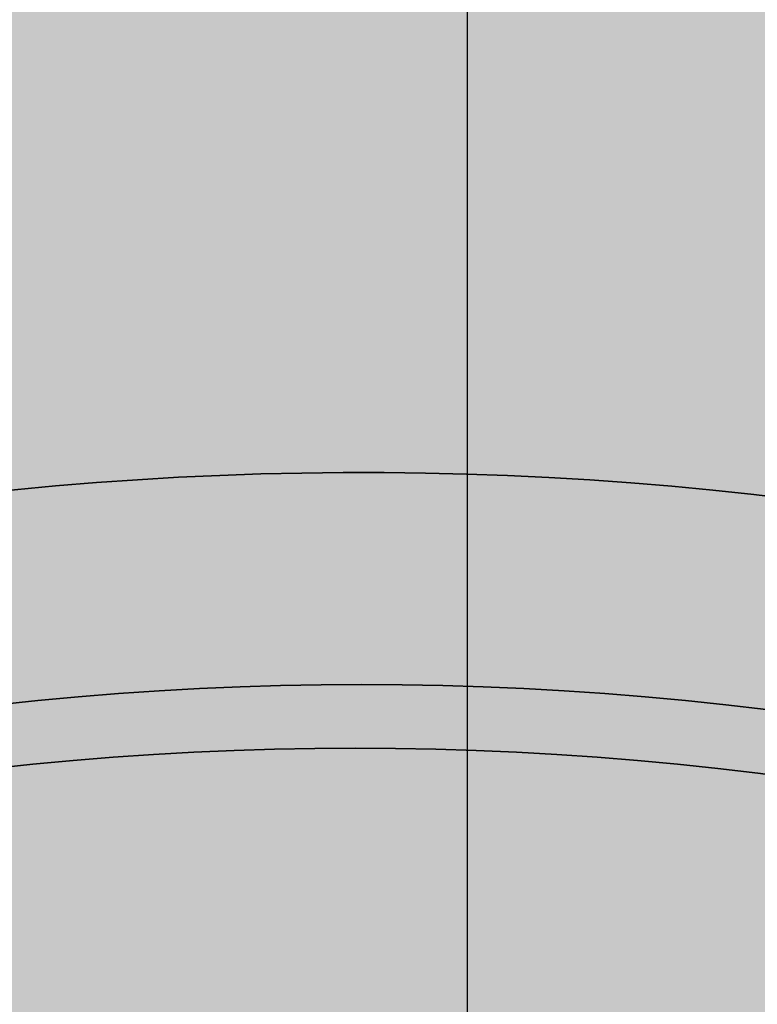
# Model space of a CAD drawing. Units: millimetres. Extents: x 130 to 1021, y 147 to 699.
# Tile 7 of 40: x 411 to 446, y 394 to 440. Entities that reach past the tile are written whole.
import ezdxf

# ---------------------------------------------------------------- set-up
doc = ezdxf.new("R2010")
doc.units = ezdxf.units.MM
doc.header["$MEASUREMENT"] = 0
for name, color, linetype, lineweight in [('A-ANNO-DIMS', 2, 'Continuous', 18), ('A-ELEV', 7, 'Continuous', 35), ('A-ELEV-PATT', 9, 'Continuous', 13)]:
    doc.layers.add(name, color=color, linetype=linetype, lineweight=lineweight)
doc.styles.get("Standard").update_dxf_attribs({"font": 'arial.ttf'})
doc.dimstyles.get("Standard").update_dxf_attribs({"dimtxt": 20, "dimasz": 10, "dimexe": 10, "dimexo": 10, "dimgap": 5, "dimtad": 0, "dimtih": 1, "dimtoh": 1, "dimdec": 0, "dimzin": 0, "dimdsep": 46, "dimtxsty": 'Standard', "dimcen": 5, "dimadec": 0, "dimazin": 0, "dimtfac": 1, "dimtdec": 0, "dimtofl": 0, "dimtmove": 0, "dimatfit": 3, "dimfxl": 1, "dimtolj": 1, "dimtzin": 0, "dimarcsym": 0})

# ---------------------------------------------------------------- blocks, each defined once
blk = doc.blocks.new('*D7')
at = {"layer": 'A-ANNO-DIMS', "color": 0, "lineweight": -2, "transparency": 16777216}
for p, q in [((399.374, 349.447), (413.374, 349.447)), ((423.374, 349.447), (433.374, 349.447)), ((389.374, 344.547), (389.374, 339.447)), ((423.374, 344.547), (423.374, 339.447))]:
    blk.add_line(p, q, dxfattribs=at)
at = {"layer": 'A-ANNO-DIMS', "color": 0, "transparency": 16777216}
for points in [[(399.374, 351.114), (399.374, 347.781), (389.374, 349.447)], [(413.374, 351.114), (413.374, 347.781), (423.374, 349.447)]]:
    blk.add_solid(points, dxfattribs=at)
at = {"layer": 'Defpoints', "color": 0, "transparency": 16777216}
for p in [(389.374, 354.547), (423.374, 354.547), (423.374, 349.447)]:
    blk.add_point(p, dxfattribs=at)
at = {"layer": 'A-ANNO-DIMS', "color": 0, "transparency": 16777216, "insert": (582.037, 349.447), "char_height": 20, "attachment_point": 5}
blk.add_mtext('\\A1;DOOR PANEL 34 TYP.', dxfattribs=at)
blk = doc.blocks.new('*D8')
at = {"layer": 'A-ANNO-DIMS', "color": 0, "lineweight": -2, "transparency": 16777216}
for p, q in [((428.474, 380.947), (428.474, 390.947)), ((428.474, 390.947), (438.474, 390.947)), ((433.374, 370.947), (438.474, 370.947)), ((433.374, 354.547), (438.474, 354.547)), ((428.474, 344.547), (428.474, 334.547))]:
    blk.add_line(p, q, dxfattribs=at)
at = {"layer": 'A-ANNO-DIMS', "color": 0, "transparency": 16777216}
for points in [[(426.807, 380.947), (430.14, 380.947), (428.474, 370.947)], [(426.807, 344.547), (430.14, 344.547), (428.474, 354.547)]]:
    blk.add_solid(points, dxfattribs=at)
at = {"layer": 'Defpoints', "color": 0, "transparency": 16777216}
for p in [(423.374, 370.947), (428.474, 370.947), (423.374, 354.547)]:
    blk.add_point(p, dxfattribs=at)
at = {"layer": 'A-ANNO-DIMS', "color": 0, "transparency": 16777216, "insert": (491.209, 390.947), "char_height": 20, "attachment_point": 5}
blk.add_mtext('\\A1;16 TYP.', dxfattribs=at)
blk = doc.blocks.new('*D11')
at = {"layer": 'A-ANNO-DIMS', "color": 0, "lineweight": -2, "transparency": 16777216}
for p, q in [((737.374, 648.699), (737.374, 149.739)), ((299.374, 566.947), (299.374, 149.739)), ((309.374, 159.739), (490.857, 159.739)), ((727.374, 159.739), (545.891, 159.739))]:
    blk.add_line(p, q, dxfattribs=at)
at = {"layer": 'A-ANNO-DIMS', "color": 0, "transparency": 16777216}
for points in [[(309.374, 161.406), (309.374, 158.073), (299.374, 159.739)], [(727.374, 161.406), (727.374, 158.073), (737.374, 159.739)]]:
    blk.add_solid(points, dxfattribs=at)
at = {"layer": 'Defpoints', "color": 0, "transparency": 16777216}
for p in [(737.374, 658.699), (299.374, 576.947), (737.374, 159.739)]:
    blk.add_point(p, dxfattribs=at)
at = {"layer": 'A-ANNO-DIMS', "color": 0, "transparency": 16777216, "insert": (518.374, 159.739), "char_height": 20, "attachment_point": 5}
blk.add_mtext('\\A1;438', dxfattribs=at)
blk = doc.blocks.new('*D12')
at = {"layer": 'A-ANNO-DIMS', "color": 0, "lineweight": -2, "transparency": 16777216}
for p, q in [((477.374, 661.947), (265.074, 661.947)), ((275.074, 651.947), (275.074, 438.205)), ((275.074, 194.039), (275.074, 407.782)), ((357.163, 184.039), (265.074, 184.039))]:
    blk.add_line(p, q, dxfattribs=at)
at = {"layer": 'A-ANNO-DIMS', "color": 0, "transparency": 16777216}
for points in [[(273.407, 651.947), (276.74, 651.947), (275.074, 661.947)], [(273.407, 194.039), (276.74, 194.039), (275.074, 184.039)]]:
    blk.add_solid(points, dxfattribs=at)
at = {"layer": 'Defpoints', "color": 0, "transparency": 16777216}
for p in [(275.074, 661.947), (487.374, 661.947), (367.163, 184.039)]:
    blk.add_point(p, dxfattribs=at)
at = {"layer": 'A-ANNO-DIMS', "color": 0, "transparency": 16777216, "insert": (275.074, 422.993), "char_height": 20, "attachment_point": 5}
blk.add_mtext('\\A1;477.9', dxfattribs=at)
blk = doc.blocks.new('*D15')
at = {"layer": 'A-ANNO-DIMS', "color": 0, "lineweight": -2, "transparency": 16777216}
for p, q in [((327.374, 579.884), (327.374, 696.247)), ((357.941, 411.947), (357.941, 696.247)), ((337.374, 686.247), (347.941, 686.247)), ((357.941, 686.247), (367.941, 686.247))]:
    blk.add_line(p, q, dxfattribs=at)
at = {"layer": 'A-ANNO-DIMS', "color": 0, "transparency": 16777216}
for points in [[(337.374, 687.914), (337.374, 684.581), (327.374, 686.247)], [(347.941, 687.914), (347.941, 684.581), (357.941, 686.247)]]:
    blk.add_solid(points, dxfattribs=at)
at = {"layer": 'Defpoints', "color": 0, "transparency": 16777216}
for p in [(357.941, 686.247), (327.374, 569.884), (357.941, 401.947)]:
    blk.add_point(p, dxfattribs=at)
at = {"layer": 'A-ANNO-DIMS', "color": 0, "transparency": 16777216, "insert": (406.679, 686.247), "char_height": 20, "attachment_point": 5}
blk.add_mtext('\\A1;30.57', dxfattribs=at)
blk = doc.blocks.new('*D16')
at = {"layer": 'A-ANNO-DIMS', "color": 0, "lineweight": -2, "transparency": 16777216}
for p, q in [((357.941, 411.947), (357.941, 696.247)), ((363.922, 579.884), (363.922, 696.247)), ((347.941, 686.247), (337.941, 686.247)), ((373.922, 686.247), (383.922, 686.247))]:
    blk.add_line(p, q, dxfattribs=at)
at = {"layer": 'A-ANNO-DIMS', "color": 0, "transparency": 16777216}
for points in [[(347.941, 687.914), (347.941, 684.581), (357.941, 686.247)], [(373.922, 687.914), (373.922, 684.581), (363.922, 686.247)]]:
    blk.add_solid(points, dxfattribs=at)
at = {"layer": 'Defpoints', "color": 0, "transparency": 16777216}
for p in [(363.922, 686.247), (363.922, 569.884), (357.941, 401.947)]:
    blk.add_point(p, dxfattribs=at)
at = {"layer": 'A-ANNO-DIMS', "color": 0, "transparency": 16777216, "insert": (420.737, 686.247), "char_height": 20, "attachment_point": 5}
blk.add_mtext('\\A1;5.981', dxfattribs=at)
blk = doc.blocks.new('*D18')
at = {"layer": 'A-ANNO-DIMS', "color": 0, "lineweight": -2, "transparency": 16777216}
for p, q in [((375.85, 490.216), (375.85, 696.247)), ((382.374, 388.947), (382.374, 696.247)), ((365.85, 686.247), (355.85, 686.247)), ((392.374, 686.247), (402.374, 686.247))]:
    blk.add_line(p, q, dxfattribs=at)
at = {"layer": 'A-ANNO-DIMS', "color": 0, "transparency": 16777216}
for points in [[(365.85, 687.914), (365.85, 684.581), (375.85, 686.247)], [(392.374, 687.914), (392.374, 684.581), (382.374, 686.247)]]:
    blk.add_solid(points, dxfattribs=at)
at = {"layer": 'Defpoints', "color": 0, "transparency": 16777216}
for p in [(382.374, 686.247), (375.85, 480.216), (382.374, 378.947)]:
    blk.add_point(p, dxfattribs=at)
at = {"layer": 'A-ANNO-DIMS', "color": 0, "transparency": 16777216, "insert": (441.132, 686.247), "char_height": 20, "attachment_point": 5}
blk.add_mtext('\\A1;6.524', dxfattribs=at)
blk = doc.blocks.new('*D19')
at = {"layer": 'A-ANNO-DIMS', "color": 0, "lineweight": -2, "transparency": 16777216}
for p, q in [((382.374, 388.947), (382.374, 696.247)), ((414.652, 510.881), (414.652, 696.247)), ((392.374, 686.247), (404.652, 686.247)), ((414.652, 686.247), (424.652, 686.247))]:
    blk.add_line(p, q, dxfattribs=at)
at = {"layer": 'A-ANNO-DIMS', "color": 0, "transparency": 16777216}
for points in [[(392.374, 687.914), (392.374, 684.581), (382.374, 686.247)], [(404.652, 687.914), (404.652, 684.581), (414.652, 686.247)]]:
    blk.add_solid(points, dxfattribs=at)
at = {"layer": 'Defpoints', "color": 0, "transparency": 16777216}
for p in [(414.652, 686.247), (414.652, 500.881), (382.374, 378.947)]:
    blk.add_point(p, dxfattribs=at)
at = {"layer": 'A-ANNO-DIMS', "color": 0, "transparency": 16777216, "insert": (463.411, 686.247), "char_height": 20, "attachment_point": 5}
blk.add_mtext('\\A1;32.28', dxfattribs=at)
blk = doc.blocks.new('*D20')
at = {"layer": 'A-ANNO-DIMS', "color": 0, "lineweight": -2, "transparency": 16777216}
for p, q in [((414.652, 510.881), (414.652, 696.247)), ((432.374, 388.947), (432.374, 696.247)), ((404.652, 686.247), (394.652, 686.247)), ((442.374, 686.247), (452.374, 686.247))]:
    blk.add_line(p, q, dxfattribs=at)
at = {"layer": 'A-ANNO-DIMS', "color": 0, "transparency": 16777216}
for points in [[(404.652, 687.914), (404.652, 684.581), (414.652, 686.247)], [(442.374, 687.914), (442.374, 684.581), (432.374, 686.247)]]:
    blk.add_solid(points, dxfattribs=at)
at = {"layer": 'Defpoints', "color": 0, "transparency": 16777216}
for p in [(432.374, 686.247), (414.652, 500.881), (432.374, 378.947)]:
    blk.add_point(p, dxfattribs=at)
at = {"layer": 'A-ANNO-DIMS', "color": 0, "transparency": 16777216, "insert": (490.075, 686.247), "char_height": 20, "attachment_point": 5}
blk.add_mtext('\\A1;17.72', dxfattribs=at)
blk = doc.blocks.new('*D21')
at = {"layer": 'A-ANNO-DIMS', "color": 0, "lineweight": -2, "transparency": 16777216}
for p, q in [((432.374, 388.947), (432.374, 696.247)), ((447.374, 656.947), (447.374, 696.247)), ((422.374, 686.247), (412.374, 686.247)), ((457.374, 686.247), (467.374, 686.247))]:
    blk.add_line(p, q, dxfattribs=at)
at = {"layer": 'A-ANNO-DIMS', "color": 0, "transparency": 16777216}
for points in [[(422.374, 687.914), (422.374, 684.581), (432.374, 686.247)], [(457.374, 687.914), (457.374, 684.581), (447.374, 686.247)]]:
    blk.add_solid(points, dxfattribs=at)
at = {"layer": 'Defpoints', "color": 0, "transparency": 16777216}
for p in [(447.374, 686.247), (447.374, 646.947), (432.374, 378.947)]:
    blk.add_point(p, dxfattribs=at)
at = {"layer": 'A-ANNO-DIMS', "color": 0, "transparency": 16777216, "insert": (485.832, 686.247), "char_height": 20, "attachment_point": 5}
blk.add_mtext('\\A1;15', dxfattribs=at)
blk = doc.blocks.new('*D22')
at = {"layer": 'A-ANNO-DIMS', "color": 0, "lineweight": -2, "transparency": 16777216}
for p, q in [((447.374, 656.947), (447.374, 696.247)), ((466.767, 403.947), (466.767, 696.247)), ((437.374, 686.247), (427.374, 686.247)), ((476.767, 686.247), (486.767, 686.247))]:
    blk.add_line(p, q, dxfattribs=at)
at = {"layer": 'A-ANNO-DIMS', "color": 0, "transparency": 16777216}
for points in [[(437.374, 687.914), (437.374, 684.581), (447.374, 686.247)], [(476.767, 687.914), (476.767, 684.581), (466.767, 686.247)]]:
    blk.add_solid(points, dxfattribs=at)
at = {"layer": 'Defpoints', "color": 0, "transparency": 16777216}
for p in [(466.767, 686.247), (447.374, 646.947), (466.767, 393.947)]:
    blk.add_point(p, dxfattribs=at)
at = {"layer": 'A-ANNO-DIMS', "color": 0, "transparency": 16777216, "insert": (532.34, 686.247), "char_height": 20, "attachment_point": 5}
blk.add_mtext('\\A1;19.393', dxfattribs=at)
blk = doc.blocks.new('*D64')
at = {"layer": 'A-ANNO-DIMS', "color": 0, "lineweight": -2, "transparency": 16777216}
for p, q in [((502.049, 450.926), (502.049, 460.926)), ((497.049, 455.926), (507.049, 455.926)), ((363.96, 263.061), (409.922, 327.255)), ((353.96, 263.061), (363.96, 263.061))]:
    blk.add_line(p, q, dxfattribs=at)
at = {"layer": 'A-ANNO-DIMS', "color": 0, "transparency": 16777216}
blk.add_solid([(408.567, 328.225), (411.277, 326.284), (415.743, 335.385)], dxfattribs=at)
at = {"layer": 'Defpoints', "color": 0, "transparency": 16777216}
for p in [(502.049, 455.926), (415.743, 335.385)]:
    blk.add_point(p, dxfattribs=at)
at = {"layer": 'A-ANNO-DIMS', "color": 0, "transparency": 16777216, "insert": (297.8, 263.061), "char_height": 20, "attachment_point": 5}
blk.add_mtext('\\A1;R148.25', dxfattribs=at)
blk = doc.blocks.new('*D65')
at = {"layer": 'A-ANNO-DIMS', "color": 0, "lineweight": -2, "transparency": 16777216}
for p, q in [((495.463, 509.127), (472.508, 423.108)), ((505.463, 509.127), (495.463, 509.127)), ((427.374, 248.979), (427.374, 258.979)), ((422.374, 253.979), (432.374, 253.979))]:
    blk.add_line(p, q, dxfattribs=at)
at = {"layer": 'A-ANNO-DIMS', "color": 0, "transparency": 16777216}
blk.add_solid([(470.898, 423.538), (474.118, 422.679), (469.93, 413.447)], dxfattribs=at)
at = {"layer": 'Defpoints', "color": 0, "transparency": 16777216}
for p in [(469.93, 413.447), (427.374, 253.979)]:
    blk.add_point(p, dxfattribs=at)
at = {"layer": 'A-ANNO-DIMS', "color": 0, "transparency": 16777216, "insert": (561.623, 509.127), "char_height": 20, "attachment_point": 5}
blk.add_mtext('\\A1;R165.05', dxfattribs=at)
blk = doc.blocks.new('*D66')
at = {"layer": 'A-ANNO-DIMS', "color": 0, "lineweight": -2, "transparency": 16777216}
for p, q in [((341.579, 557.194), (351.579, 557.194)), ((351.579, 557.194), (376.947, 478.135)), ((427.374, 315.978), (427.374, 325.978)), ((422.374, 320.978), (432.374, 320.978))]:
    blk.add_line(p, q, dxfattribs=at)
at = {"layer": 'A-ANNO-DIMS', "color": 0, "transparency": 16777216}
blk.add_solid([(378.534, 478.644), (375.36, 477.626), (380.002, 468.613)], dxfattribs=at)
at = {"layer": 'Defpoints', "color": 0, "transparency": 16777216}
for p in [(380.002, 468.613), (427.374, 320.978)]:
    blk.add_point(p, dxfattribs=at)
at = {"layer": 'A-ANNO-DIMS', "color": 0, "transparency": 16777216, "insert": (263.53, 557.194), "char_height": 20, "attachment_point": 5}
blk.add_mtext('\\A1;4X R155.05', dxfattribs=at)
blk = doc.blocks.new('*D67')
at = {"layer": 'A-ANNO-DIMS', "color": 0, "lineweight": -2, "transparency": 16777216}
for p, q in [((479.756, 492.431), (462.144, 412.223)), ((489.756, 492.431), (479.756, 492.431)), ((427.07, 247.496), (427.07, 257.496)), ((422.07, 252.496), (432.07, 252.496))]:
    blk.add_line(p, q, dxfattribs=at)
at = {"layer": 'A-ANNO-DIMS', "color": 0, "transparency": 16777216}
blk.add_solid([(460.516, 412.58), (463.772, 411.865), (459.999, 402.455)], dxfattribs=at)
at = {"layer": 'Defpoints', "color": 0, "transparency": 16777216}
for p in [(459.999, 402.455), (427.07, 252.496)]:
    blk.add_point(p, dxfattribs=at)
at = {"layer": 'A-ANNO-DIMS', "color": 0, "transparency": 16777216, "insert": (545.841, 492.431), "char_height": 20, "attachment_point": 5}
blk.add_mtext('\\A1;R153.53', dxfattribs=at)
blk = doc.blocks.new('*D68')
at = {"layer": 'A-ANNO-DIMS', "color": 0, "lineweight": -2, "transparency": 16777216}
for p, q in [((361.841, 579.756), (371.841, 579.756)), ((371.841, 579.756), (392.167, 506.693)), ((433.191, 354.23), (433.191, 364.23)), ((428.191, 359.23), (438.191, 359.23))]:
    blk.add_line(p, q, dxfattribs=at)
at = {"layer": 'A-ANNO-DIMS', "color": 0, "transparency": 16777216}
blk.add_solid([(393.773, 507.14), (390.561, 506.246), (394.847, 497.059)], dxfattribs=at)
at = {"layer": 'Defpoints', "color": 0, "transparency": 16777216}
for p in [(394.847, 497.059), (433.191, 359.23)]:
    blk.add_point(p, dxfattribs=at)
at = {"layer": 'A-ANNO-DIMS', "color": 0, "transparency": 16777216, "insert": (305.764, 579.756), "char_height": 20, "attachment_point": 5}
blk.add_mtext('\\A1;R143.06', dxfattribs=at)
blk = doc.blocks.new('*D69')
at = {"layer": 'A-ANNO-DIMS', "color": 0, "lineweight": -2, "transparency": 16777216}
for p, q in [((507.746, 572.261), (483.091, 501.813)), ((517.746, 572.261), (507.746, 572.261)), ((433.191, 354.23), (433.191, 364.23)), ((428.191, 359.23), (438.191, 359.23))]:
    blk.add_line(p, q, dxfattribs=at)
at = {"layer": 'A-ANNO-DIMS', "color": 0, "transparency": 16777216}
blk.add_solid([(481.518, 502.363), (484.664, 501.262), (479.788, 492.374)], dxfattribs=at)
at = {"layer": 'Defpoints', "color": 0, "transparency": 16777216}
for p in [(479.788, 492.374), (433.191, 359.23)]:
    blk.add_point(p, dxfattribs=at)
at = {"layer": 'A-ANNO-DIMS', "color": 0, "transparency": 16777216, "insert": (573.824, 572.261), "char_height": 20, "attachment_point": 5}
blk.add_mtext('\\A1;R141.06', dxfattribs=at)
blk = doc.blocks.new('*D70')
at = {"layer": 'A-ANNO-DIMS', "color": 0, "lineweight": -2, "transparency": 16777216}
for p, q in [((370.141, 588.4), (380.141, 588.4)), ((380.141, 588.4), (397.473, 517.008)), ((432.65, 367.109), (432.65, 377.109)), ((427.65, 372.109), (437.65, 372.109))]:
    blk.add_line(p, q, dxfattribs=at)
at = {"layer": 'A-ANNO-DIMS', "color": 0, "transparency": 16777216}
blk.add_solid([(399.093, 517.402), (395.854, 516.615), (399.832, 507.291)], dxfattribs=at)
at = {"layer": 'Defpoints', "color": 0, "transparency": 16777216}
for p in [(399.832, 507.291), (432.65, 372.109)]:
    blk.add_point(p, dxfattribs=at)
at = {"layer": 'A-ANNO-DIMS', "color": 0, "transparency": 16777216, "insert": (323.757, 588.4), "char_height": 20, "attachment_point": 5}
blk.add_mtext('\\A1;R139.1', dxfattribs=at)
blk = doc.blocks.new('*D71')
at = {"layer": 'A-ANNO-DIMS', "color": 0, "lineweight": -2, "transparency": 16777216}
for p, q in [((492.108, 581.609), (472.542, 512.666)), ((502.108, 581.609), (492.108, 581.609)), ((432.65, 367.109), (432.65, 377.109)), ((427.65, 372.109), (437.65, 372.109))]:
    blk.add_line(p, q, dxfattribs=at)
at = {"layer": 'A-ANNO-DIMS', "color": 0, "transparency": 16777216}
blk.add_solid([(470.938, 513.121), (474.145, 512.211), (469.812, 503.046)], dxfattribs=at)
at = {"layer": 'Defpoints', "color": 0, "transparency": 16777216}
for p in [(469.812, 503.046), (432.65, 372.109)]:
    blk.add_point(p, dxfattribs=at)
at = {"layer": 'A-ANNO-DIMS', "color": 0, "transparency": 16777216, "insert": (548.493, 581.609), "char_height": 20, "attachment_point": 5}
blk.add_mtext('\\A1;R136.1', dxfattribs=at)
blk = doc.blocks.new('*D72')
at = {"layer": 'A-ANNO-DIMS', "color": 0, "lineweight": -2, "transparency": 16777216}
for p, q in [((460.658, 573.64), (451.279, 503.49)), ((470.658, 573.64), (460.658, 573.64)), ((432.115, 355.142), (432.115, 365.142)), ((427.115, 360.142), (437.115, 360.142))]:
    blk.add_line(p, q, dxfattribs=at)
at = {"layer": 'A-ANNO-DIMS', "color": 0, "transparency": 16777216}
blk.add_solid([(449.628, 503.711), (452.931, 503.27), (449.954, 493.579)], dxfattribs=at)
at = {"layer": 'Defpoints', "color": 0, "transparency": 16777216}
for p in [(449.954, 493.579), (432.115, 360.142)]:
    blk.add_point(p, dxfattribs=at)
at = {"layer": 'A-ANNO-DIMS', "color": 0, "transparency": 16777216, "insert": (526.64, 573.64), "char_height": 20, "attachment_point": 5}
blk.add_mtext('\\A1;R134.62', dxfattribs=at)
blk = doc.blocks.new('*D73')
at = {"layer": 'A-ANNO-DIMS', "color": 0, "lineweight": -2, "transparency": 16777216}
for p, q in [((402.678, 571.448), (412.678, 571.448)), ((412.678, 571.448), (419.051, 502.166)), ((432.115, 355.142), (432.115, 365.142)), ((427.115, 360.142), (437.115, 360.142))]:
    blk.add_line(p, q, dxfattribs=at)
at = {"layer": 'A-ANNO-DIMS', "color": 0, "transparency": 16777216}
blk.add_solid([(420.711, 502.319), (417.391, 502.014), (419.967, 492.208)], dxfattribs=at)
at = {"layer": 'Defpoints', "color": 0, "transparency": 16777216}
for p in [(419.967, 492.208), (432.115, 360.142)]:
    blk.add_point(p, dxfattribs=at)
at = {"layer": 'A-ANNO-DIMS', "color": 0, "transparency": 16777216, "insert": (346.696, 571.448), "char_height": 20, "attachment_point": 5}
blk.add_mtext('\\A1;R132.62', dxfattribs=at)

msp = doc.modelspace()

# ---------------------------------------------------------------- hatches: boundary and pattern name
at = {"layer": 'A-ELEV-PATT'}
h = msp.add_hatch(color=256, dxfattribs=at)
h.dxf.hatch_style = 1
h.paths.add_polyline_path([(737.3738, 658.6988, 0.0135961), (632.4019, 661.9473), (607.3738, 661.9473), (487.3738, 661.9473), (487.3738, 649.9473), (607.3738, 649.9473), (632.3794, 649.9473, -0.0136841), (737.3738, 646.6784)])
h.paths.add_polyline_path([(732.3738, 643.9599, 0.0130529), (632.3738, 646.9473), (607.3738, 646.9473), (487.3738, 646.9473), (487.3738, 596.9473), (632.3738, 596.9473, -0.0130529), (732.3738, 593.9599)])
h.paths.add_polyline_path([(737.3738, 593.6732, 0.0137063), (632.3738, 596.9473), (487.3738, 596.9473), (487.3738, 586.9473), (632.355, 586.9473, -0.0137808), (737.3738, 583.6559)])
h.paths.add_polyline_path([(447.3738, 646.9473), (307.3738, 646.9473), (302.3738, 646.9473), (302.3738, 634.9473), (447.3738, 634.9473)])
h.paths.add_polyline_path([(447.3738, 631.9473), (307.3738, 631.9473), (307.3738, 586.9473), (447.3738, 586.9473)])
h.paths.add_polyline_path([(447.3738, 586.9473), (307.3738, 586.9473), (302.3738, 586.9473), (302.3738, 576.9473), (447.3738, 576.9473)])
h.paths.add_polyline_path([(447.3738, 573.9473), (367.3738, 573.9473), (367.3738, 539.9473), (447.3738, 539.9473)])
h.paths.add_polyline_path([(447.3738, 537.9473), (367.3738, 537.9473), (367.3738, 507.9473), (400.392, 507.4253, -0.001728), (401.3281, 507.6451, -0.5220025), (425.6117, 511.0391, -0.0391849), (447.3738, 510.4359), (447.3738, 510.7883)])
h.paths.add_polyline_path([(394.7238, 505.9473), (367.3738, 505.9473), (367.3738, 476.9473, -0.0146512), (375.8501, 480.2159), (376.1506, 499.2266, -0.0355419)])
h.paths.add_polyline_path([(632.3738, 583.9473), (552.3738, 583.9473), (552.3738, 550.9473), (632.3738, 550.9473)])
h.paths.add_polyline_path([(632.3738, 548.9473), (552.3738, 548.9473), (552.3738, 515.9473), (632.3738, 515.9473)])
h.paths.add_polyline_path([(632.3738, 513.9473), (552.3738, 513.9473), (552.3738, 476.9473), (632.3738, 476.9473)])
h.paths.add_polyline_path([(737.3738, 473.6903, 0.0136326), (632.3926, 476.9473), (552.3738, 476.9473), (487.3738, 476.9473), (487.3738, 466.9473), (632.3738, 466.9473, -0.0137063), (737.3738, 463.6732)])
h.paths.add_polyline_path([(732.3738, 460.9552, 0.0130741), (632.3681, 463.9473), (487.3738, 463.9473), (487.3738, 407.735, -0.0032286), (489.3544, 406.9473), (632.3926, 406.9473, -0.0129826), (732.3738, 403.9755)])
h.paths.add_polyline_path([(487.3738, 463.9473, 0.20133), (367.3738, 463.9473), (367.3738, 407.735, -0.1882031), (487.3738, 407.735)])
h.paths.add_polyline_path([(367.3738, 476.9473), (367.3738, 466.9473, -0.2013309), (487.3738, 466.9473), (487.3738, 476.9473, 0.20133)])
h.paths.add_polyline_path([(367.3738, 463.9473), (307.3738, 463.9473), (307.3738, 401.9473), (357.9413, 401.9473), (367.3738, 407.735)])
h.paths.add_polyline_path([(367.3738, 476.9473), (302.3738, 476.9473), (302.3738, 466.9473), (367.3738, 466.9473)])
h.paths.add_polyline_path([(632.8184, 366.9453), (552.3738, 366.9453), (552.3738, 393.9473), (632.8184, 393.9473)])
h.paths.add_polyline_path([(632.8184, 357.2114), (632.8184, 363.9453), (552.3738, 363.9453), (552.3738, 357.2114), (552.3738, 336.9453), (632.8184, 336.9453)])
h.paths.add_polyline_path([(632.8184, 333.9453), (552.3738, 333.9453), (552.3738, 306.9453), (632.8184, 306.9453)])
h.paths.add_polyline_path([(632.8184, 303.9453), (552.3738, 303.9453), (552.3738, 273.9473), (632.355, 273.9473, 0.0000608), (632.8184, 273.9491)])
h.paths.add_polyline_path([(737.3738, 403.6903, 0.0136326), (632.3926, 406.9473), (489.3544, 406.9473, 0.1915481), (367.3738, 407.735), (367.3738, 396.9473, -0.2013309), (487.3738, 396.9473), (632.3738, 396.9473, -0.0137063), (737.3738, 393.6732)])
h.paths.add_polyline_path([(357.9413, 401.9473), (307.3738, 401.9473), (307.3738, 391.9473), (357.9413, 391.9473)])
h.paths.add_polyline_path([(357.9413, 357.2114), (357.9413, 388.9473), (307.3738, 388.9473), (307.3738, 357.2114), (307.3738, 273.9473), (357.9413, 273.9473)])
h.paths.add_polyline_path([(732.3738, 263.93, -0.0130317), (632.3794, 260.9473), (466.7667, 260.9473), (466.7667, 240.9473), (469.8406, 236.978), (469.8406, 221.978), (472.9145, 218.0087), (472.9145, 213.9473), (607.3738, 213.9473), (732.3738, 213.9473)])
h.paths.add_polyline_path([(732.3738, 290.889), (722.479, 290.889), (722.479, 301.889), (732.3738, 301.889), (732.3738, 305.889), (722.479, 305.889), (722.479, 316.889), (732.3738, 316.889), (732.3738, 320.889), (722.479, 320.889), (722.479, 331.889), (732.3738, 331.889), (732.3738, 335.889), (722.479, 335.889), (722.479, 346.889), (732.3738, 346.889), (732.3738, 350.889), (722.479, 350.889), (722.479, 361.889), (732.3738, 361.889), (732.3738, 365.889), (722.479, 365.889), (722.479, 376.889), (732.3738, 376.889), (732.3738, 380.889), (722.479, 380.889), (722.479, 391.4848, 0.0005233), (718.479, 391.6843), (718.479, 380.889), (707.479, 380.889), (707.479, 392.1896, 0.0005231), (703.479, 392.3576), (703.479, 380.889), (692.479, 380.889), (692.479, 392.7765, 0.0005229), (688.479, 392.9131), (688.479, 380.889), (677.479, 380.889), (677.479, 393.2456, 0.0005228), (673.479, 393.3508), (673.479, 380.889), (662.479, 380.889), (662.479, 393.597, 0.0005227), (658.479, 393.6709), (658.479, 380.889), (647.479, 380.889), (647.479, 393.8308, 0.0005226), (643.479, 393.8732), (643.479, 380.889), (632.8184, 380.889), (632.8184, 376.889), (643.479, 376.889), (643.479, 365.889), (632.8184, 365.889), (632.8184, 361.889), (643.479, 361.889), (643.479, 350.889), (632.8184, 350.889), (632.8184, 346.889), (643.479, 346.889), (643.479, 335.889), (632.8184, 335.889), (632.8184, 331.889), (643.479, 331.889), (643.479, 320.889), (632.8184, 320.889), (632.8184, 316.889), (643.479, 316.889), (643.479, 305.889), (632.8184, 305.889), (632.8184, 301.889), (643.479, 301.889), (643.479, 290.889), (632.8184, 290.889), (632.8184, 286.889), (643.479, 286.889), (643.479, 274.0217, 0.0005246), (647.479, 274.0643), (647.479, 286.889), (658.479, 286.889), (658.479, 274.2248, 0.0005246), (662.479, 274.2989), (662.479, 286.889), (673.479, 286.889), (673.479, 274.546, 0.0005247), (677.479, 274.6516), (677.479, 286.889), (688.479, 286.889), (688.479, 274.9853, 0.0005248), (692.479, 275.1224), (692.479, 286.889), (703.479, 286.889), (703.479, 275.5429, 0.000525), (707.479, 275.7115), (707.479, 286.889), (718.479, 286.889), (718.479, 276.2187, 0.0005252), (722.479, 276.4189), (722.479, 286.889), (732.3738, 286.889)])
h.paths.add_polyline_path([(718.479, 290.889), (707.479, 290.889), (707.479, 301.889), (718.479, 301.889)], flags=16)
h.paths.add_polyline_path([(703.479, 290.889), (692.479, 290.889), (692.479, 301.889), (703.479, 301.889)], flags=16)
h.paths.add_polyline_path([(718.479, 305.889), (707.479, 305.889), (707.479, 316.889), (718.479, 316.889)], flags=16)
h.paths.add_polyline_path([(703.479, 305.889), (692.479, 305.889), (692.479, 316.889), (703.479, 316.889)], flags=16)
h.paths.add_polyline_path([(688.479, 290.889), (677.479, 290.889), (677.479, 301.889), (688.479, 301.889)], flags=16)
h.paths.add_polyline_path([(718.479, 320.889), (707.479, 320.889), (707.479, 331.889), (718.479, 331.889)], flags=16)
h.paths.add_polyline_path([(688.479, 305.889), (677.479, 305.889), (677.479, 316.889), (688.479, 316.889)], flags=16)
h.paths.add_polyline_path([(703.479, 320.889), (692.479, 320.889), (692.479, 331.889), (703.479, 331.889)], flags=16)
h.paths.add_polyline_path([(688.479, 320.889), (677.479, 320.889), (677.479, 331.889), (688.479, 331.889)], flags=16)
h.paths.add_polyline_path([(673.479, 290.889), (662.479, 290.889), (662.479, 301.889), (673.479, 301.889)], flags=16)
h.paths.add_polyline_path([(718.479, 335.889), (707.479, 335.889), (707.479, 346.889), (718.479, 346.889)], flags=16)
h.paths.add_polyline_path([(673.479, 305.889), (662.479, 305.889), (662.479, 316.889), (673.479, 316.889)], flags=16)
h.paths.add_polyline_path([(703.479, 335.889), (692.479, 335.889), (692.479, 346.889), (703.479, 346.889)], flags=16)
h.paths.add_polyline_path([(673.479, 320.889), (662.479, 320.889), (662.479, 331.889), (673.479, 331.889)], flags=16)
h.paths.add_polyline_path([(688.479, 335.889), (677.479, 335.889), (677.479, 346.889), (688.479, 346.889)], flags=16)
h.paths.add_polyline_path([(658.479, 290.889), (647.479, 290.889), (647.479, 301.889), (658.479, 301.889)], flags=16)
h.paths.add_polyline_path([(718.479, 350.889), (707.479, 350.889), (707.479, 361.889), (718.479, 361.889)], flags=16)
h.paths.add_polyline_path([(658.479, 305.889), (647.479, 305.889), (647.479, 316.889), (658.479, 316.889)], flags=16)
h.paths.add_polyline_path([(703.479, 350.889), (692.479, 350.889), (692.479, 361.889), (703.479, 361.889)], flags=16)
h.paths.add_polyline_path([(673.479, 335.889), (662.479, 335.889), (662.479, 346.889), (673.479, 346.889)], flags=16)
h.paths.add_polyline_path([(658.479, 320.889), (647.479, 320.889), (647.479, 331.889), (658.479, 331.889)], flags=16)
h.paths.add_polyline_path([(688.479, 350.889), (677.479, 350.889), (677.479, 361.889), (688.479, 361.889)], flags=16)
h.paths.add_polyline_path([(718.479, 365.889), (707.479, 365.889), (707.479, 376.889), (718.479, 376.889)], flags=16)
h.paths.add_polyline_path([(658.479, 335.889), (647.479, 335.889), (647.479, 346.889), (658.479, 346.889)], flags=16)
h.paths.add_polyline_path([(673.479, 350.889), (662.479, 350.889), (662.479, 361.889), (673.479, 361.889)], flags=16)
h.paths.add_polyline_path([(703.479, 365.889), (692.479, 365.889), (692.479, 376.889), (703.479, 376.889)], flags=16)
h.paths.add_polyline_path([(688.479, 365.889), (677.479, 365.889), (677.479, 376.889), (688.479, 376.889)], flags=16)
h.paths.add_polyline_path([(658.479, 350.889), (647.479, 350.889), (647.479, 361.889), (658.479, 361.889)], flags=16)
h.paths.add_polyline_path([(673.479, 365.889), (662.479, 365.889), (662.479, 376.889), (673.479, 376.889)], flags=16)
h.paths.add_polyline_path([(658.479, 365.889), (647.479, 365.889), (647.479, 376.889), (658.479, 376.889)], flags=16)
h.paths.add_polyline_path([(732.3738, 503.9786), (722.3392, 503.9786), (722.3392, 514.9786), (732.3738, 514.9786), (732.3738, 518.9786), (722.3392, 518.9786), (722.3392, 529.9786), (732.3738, 529.9786), (732.3738, 533.9786), (722.3392, 533.9786), (722.3392, 544.9786), (732.3738, 544.9786), (732.3738, 546.9473), (732.3738, 548.9786), (722.3392, 548.9786), (722.3392, 559.9786), (732.3738, 559.9786), (732.3738, 563.9786), (722.3392, 563.9786), (722.3392, 574.9786), (732.3738, 574.9786), (732.3738, 578.9786), (722.3392, 578.9786), (722.3392, 581.4789, 0.000526), (718.3392, 581.6791), (718.3392, 578.9786), (707.3392, 578.9786), (707.3392, 582.1863, 0.0005258), (703.3392, 582.355), (703.3392, 578.9786), (692.3392, 578.9786), (692.3392, 582.7752, 0.0005257), (688.3392, 582.9123), (688.3392, 578.9786), (677.3392, 578.9786), (677.3392, 583.2457, 0.0005255), (673.3392, 583.3512), (673.3392, 578.9786), (662.3392, 578.9786), (662.3392, 583.5978, 0.0005254), (658.3392, 583.6718), (658.3392, 578.9786), (647.3392, 578.9786), (647.3392, 583.8317, 0.0005254), (643.3392, 583.8741), (643.3392, 578.9786), (632.3738, 578.9786), (632.3738, 574.9786), (643.3392, 574.9786), (643.3392, 563.9786), (632.3738, 563.9786), (632.3738, 559.9786), (643.3392, 559.9786), (643.3392, 548.9786), (632.3738, 548.9786), (632.3738, 544.9786), (643.3392, 544.9786), (643.3392, 533.9786), (632.3738, 533.9786), (632.3738, 529.9786), (643.3392, 529.9786), (643.3392, 518.9786), (632.3738, 518.9786), (632.3738, 515.9473), (632.3738, 514.9786), (643.3392, 514.9786), (643.3392, 503.9786), (632.3738, 503.9786), (632.3738, 499.9786), (643.3392, 499.9786), (643.3392, 488.9786), (632.3738, 488.9786), (632.3738, 484.9786), (643.3392, 484.9786), (643.3392, 476.8751, -0.0005191), (647.3392, 476.8332), (647.3392, 484.9786), (658.3392, 484.9786), (658.3392, 476.6752, -0.0005192), (662.3392, 476.6022), (662.3392, 484.9786), (673.3392, 484.9786), (673.3392, 476.3585, -0.0005193), (677.3392, 476.2543), (677.3392, 484.9786), (688.3392, 484.9786), (688.3392, 475.9248, -0.0005194), (692.3392, 475.7894), (692.3392, 484.9786), (703.3392, 484.9786), (703.3392, 475.3741, -0.0005195), (707.3392, 475.2075), (707.3392, 484.9786), (718.3392, 484.9786), (718.3392, 474.7064, -0.0005197), (722.3392, 474.5086), (722.3392, 484.9786), (732.3738, 484.9786), (732.3738, 488.9786), (722.3392, 488.9786), (722.3392, 499.9786), (732.3738, 499.9786)])
h.paths.add_polyline_path([(718.3392, 503.9786), (707.3392, 503.9786), (707.3392, 514.9786), (718.3392, 514.9786)], flags=16)
h.paths.add_polyline_path([(718.3392, 499.9786), (718.3392, 488.9786), (707.3392, 488.9786), (707.3392, 499.9786)], flags=16)
h.paths.add_polyline_path([(718.3392, 518.9786), (707.3392, 518.9786), (707.3392, 529.9786), (718.3392, 529.9786)], flags=16)
h.paths.add_polyline_path([(703.3392, 503.9786), (692.3392, 503.9786), (692.3392, 514.9786), (703.3392, 514.9786)], flags=16)
h.paths.add_polyline_path([(703.3392, 499.9786), (703.3392, 488.9786), (692.3392, 488.9786), (692.3392, 499.9786)], flags=16)
h.paths.add_polyline_path([(703.3392, 518.9786), (692.3392, 518.9786), (692.3392, 529.9786), (703.3392, 529.9786)], flags=16)
h.paths.add_polyline_path([(718.3392, 533.9786), (707.3392, 533.9786), (707.3392, 544.9786), (718.3392, 544.9786)], flags=16)
h.paths.add_polyline_path([(688.3392, 503.9786), (677.3392, 503.9786), (677.3392, 514.9786), (688.3392, 514.9786)], flags=16)
h.paths.add_polyline_path([(688.3392, 499.9786), (688.3392, 488.9786), (677.3392, 488.9786), (677.3392, 499.9786)], flags=16)
h.paths.add_polyline_path([(703.3392, 533.9786), (692.3392, 533.9786), (692.3392, 544.9786), (703.3392, 544.9786)], flags=16)
h.paths.add_polyline_path([(688.3392, 518.9786), (677.3392, 518.9786), (677.3392, 529.9786), (688.3392, 529.9786)], flags=16)
h.paths.add_polyline_path([(688.3392, 533.9786), (677.3392, 533.9786), (677.3392, 544.9786), (688.3392, 544.9786)], flags=16)
h.paths.add_polyline_path([(718.3392, 548.9786), (707.3392, 548.9786), (707.3392, 559.9786), (718.3392, 559.9786)], flags=16)
h.paths.add_polyline_path([(673.3392, 503.9786), (662.3392, 503.9786), (662.3392, 514.9786), (673.3392, 514.9786)], flags=16)
h.paths.add_polyline_path([(673.3392, 499.9786), (673.3392, 488.9786), (662.3392, 488.9786), (662.3392, 499.9786)], flags=16)
h.paths.add_polyline_path([(703.3392, 548.9786), (692.3392, 548.9786), (692.3392, 559.9786), (703.3392, 559.9786)], flags=16)
h.paths.add_polyline_path([(673.3392, 518.9786), (662.3392, 518.9786), (662.3392, 529.9786), (673.3392, 529.9786)], flags=16)
h.paths.add_polyline_path([(688.3392, 548.9786), (677.3392, 548.9786), (677.3392, 559.9786), (688.3392, 559.9786)], flags=16)
h.paths.add_polyline_path([(673.3392, 533.9786), (662.3392, 533.9786), (662.3392, 544.9786), (673.3392, 544.9786)], flags=16)
h.paths.add_polyline_path([(718.3392, 563.9786), (707.3392, 563.9786), (707.3392, 574.9786), (718.3392, 574.9786)], flags=16)
h.paths.add_polyline_path([(658.3392, 503.9786), (647.3392, 503.9786), (647.3392, 514.9786), (658.3392, 514.9786)], flags=16)
h.paths.add_polyline_path([(658.3392, 499.9786), (658.3392, 488.9786), (647.3392, 488.9786), (647.3392, 499.9786)], flags=16)
h.paths.add_polyline_path([(703.3392, 563.9786), (692.3392, 563.9786), (692.3392, 574.9786), (703.3392, 574.9786)], flags=16)
h.paths.add_polyline_path([(658.3392, 518.9786), (647.3392, 518.9786), (647.3392, 529.9786), (658.3392, 529.9786)], flags=16)
h.paths.add_polyline_path([(673.3392, 548.9786), (662.3392, 548.9786), (662.3392, 559.9786), (673.3392, 559.9786)], flags=16)
h.paths.add_polyline_path([(688.3392, 563.9786), (677.3392, 563.9786), (677.3392, 574.9786), (688.3392, 574.9786)], flags=16)
h.paths.add_polyline_path([(658.3392, 533.9786), (647.3392, 533.9786), (647.3392, 544.9786), (658.3392, 544.9786)], flags=16)
h.paths.add_polyline_path([(673.3392, 563.9786), (662.3392, 563.9786), (662.3392, 574.9786), (673.3392, 574.9786)], flags=16)
h.paths.add_polyline_path([(658.3392, 548.9786), (647.3392, 548.9786), (647.3392, 559.9786), (658.3392, 559.9786)], flags=16)
h.paths.add_polyline_path([(658.3392, 563.9786), (647.3392, 563.9786), (647.3392, 574.9786), (658.3392, 574.9786)], flags=16)
h = msp.add_hatch(color=256, dxfattribs=at)
h.dxf.hatch_style = 1
h.paths.add_polyline_path([(447.3738, 576.9473), (302.3738, 576.9473), (302.3738, 573.9473), (447.3738, 573.9473)])
h.paths.add_polyline_path([(487.3738, 583.9473), (487.3738, 586.9473), (447.3738, 576.9473), (447.3738, 573.9473)])
h.paths.add_polyline_path([(632.355, 586.9473), (487.3738, 586.9473), (487.3738, 583.9473), (632.3738, 583.9473), (632.3738, 583.9472, -0.0138), (737.3738, 580.6507), (737.3738, 583.6559, 0.0137808)])
h.paths.add_polyline_path([(367.3738, 466.9473), (302.3738, 466.9473), (302.3738, 463.9473), (367.3738, 463.9473)])
h.paths.add_polyline_path([(487.3738, 463.9473), (487.3738, 466.9473, 0.2013309), (367.3738, 466.9473), (367.3738, 463.9473, -0.20133)])
h.paths.add_polyline_path([(632.3738, 466.9473), (487.3738, 466.9473), (487.3738, 463.9473), (632.3681, 463.9473, -0.0137285), (737.3738, 460.6681), (737.3738, 463.6732, 0.0137063)])
h.paths.add_polyline_path([(632.3738, 396.9473), (487.3738, 396.9473, 0.2013309), (367.3738, 396.9473), (367.3738, 393.9473, -0.2023717), (486.7667, 393.9473), (632.3681, 393.9473, -0.0137285), (737.3738, 390.6681), (737.3738, 393.6732, 0.0137063)])
h.paths.add_polyline_path([(357.9413, 391.9473), (307.3738, 391.9473), (307.3738, 388.9473), (357.9413, 388.9473)])
h.paths.add_polyline_path([(367.3738, 393.9473), (367.3738, 396.9473), (357.9413, 391.924), (357.9413, 388.9473), (358.058, 388.9473)])
h.paths.add_polyline_path([(737.3738, 264.2162), (737.3738, 267.2214, -0.0137063), (632.3738, 263.9473), (463.7667, 263.9473), (466.7667, 260.9473), (632.3794, 260.9473, 0.0136841)])
h.paths.add_polyline_path([(463.7667, 263.9473), (447.3738, 263.9473), (450.3738, 260.9473), (466.7667, 260.9473)])
h.paths.add_polyline_path([(447.3738, 263.9473), (432.3738, 263.9473), (432.3738, 260.9473), (450.3738, 260.9473)])
h.paths.add_polyline_path([(382.3738, 263.9473), (357.9413, 263.9473), (357.9413, 260.9473), (382.3738, 260.9473)])
h.paths.add_polyline_path([(357.9413, 263.9473), (307.3738, 263.9473), (307.3738, 260.9473), (357.9413, 260.9473)])
h = msp.add_hatch(color=256, dxfattribs=at)
h.dxf.hatch_style = 1
h.paths.add_polyline_path([(363.922, 569.884), (327.3738, 569.884), (327.3738, 557.9168), (363.922, 557.9168)])
h.paths.add_polyline_path([(547.7773, 577.3739), (502.3738, 577.3739), (502.3738, 566.2111), (547.7773, 566.2111)])
h.paths.add_polyline_path([(544.6354, 386.2639), (486.7667, 386.2639), (486.7667, 377.43), (544.6354, 377.43)])
h.paths.add_polyline_path([(496.0546, 377.43), (486.7667, 377.43), (486.7667, 370.4028)])
h.paths.add_polyline_path([(447.3738, 393.9473), (367.3738, 393.9473, 0.0500478), (382.3738, 368.424), (382.3738, 378.9473), (432.3738, 378.9473), (432.3738, 325.067, 0.0278945), (447.3738, 318.1243), (447.3738, 357.2114)])
h.paths.add_polyline_path([(463.5608, 388.6449), (450.8779, 388.6449), (450.8779, 363.0915), (463.5608, 363.0915)])
h.paths.add_polyline_path([(463.5608, 360.0915), (450.8779, 360.0915), (450.8779, 334.5915), (463.5608, 334.5915)])
h.paths.add_polyline_path([(463.5608, 331.5915), (450.8779, 331.5915), (450.8779, 316.785, 0.0224513), (463.5608, 312.7571)])
msp.add_hatch(color=256, dxfattribs=at).paths.add_polyline_path([(367.3738, 393.9473), (486.7667, 393.9473, 0.2023717)])

# ---------------------------------------------------------------- linework, layer by layer
at = {"layer": 'A-ELEV'}
for centre, radius, start, end in [((427.3738, 253.9788), 165.0484, 67.942927, 111.31713), ((427.3738, 253.9788), 155.0484, 67.233534, 112.766466), ((427.0702, 252.4956), 153.5326, 67.118929, 112.881071)]:
    msp.add_arc(centre, radius, start, end, dxfattribs=at)

# ---------------------------------------------------------------- dimensions: what is measured, and where the dimension line sits
at = {"layer": 'A-ANNO-DIMS'}
for base, p1, p2, override, picture, middle in [((357.9413, 686.2473), (327.3738, 569.884), (357.9413, 401.9473), {"dimdec": 2, "dimlfac": 1, "dimrnd": 0, "dimzin": 0, "dimdsep": 46, "dimlunit": 2}, '*D15', (406.6794, 686.2473)), ((363.922, 686.2473), (357.9413, 401.9473), (363.922, 569.884), {"dimdec": 3, "dimlfac": 1, "dimrnd": 0, "dimzin": 0, "dimdsep": 46, "dimlunit": 2}, '*D16', (420.7365, 686.2473)), ((382.3738, 686.2473), (375.8501, 480.2159), (382.3738, 378.9473), {"dimdec": 3, "dimlfac": 1, "dimrnd": 0, "dimzin": 0, "dimdsep": 46, "dimlunit": 2}, '*D18', (441.1323, 686.2473)), ((414.6525, 686.2473), (382.3738, 378.9473), (414.6525, 500.8811), {"dimdec": 2, "dimlfac": 1, "dimrnd": 0, "dimzin": 0, "dimdsep": 46, "dimlunit": 2}, '*D19', (463.411, 686.2473)), ((432.3738, 686.2473), (414.6525, 500.8811), (432.3738, 378.9473), {"dimdec": 2, "dimlfac": 1, "dimrnd": 0, "dimzin": 0, "dimdsep": 46, "dimlunit": 2}, '*D20', (490.075, 686.2473)), ((447.3738, 686.2473), (432.3738, 378.9473), (447.3738, 646.9473), {"dimdec": 0, "dimlfac": 1, "dimrnd": 0, "dimzin": 0, "dimdsep": 46, "dimlunit": 2}, '*D21', (485.8322, 686.2473)), ((466.7667, 686.2473), (447.3738, 646.9473), (466.7667, 393.9473), {"dimdec": 3, "dimlfac": 1, "dimrnd": 0, "dimzin": 0, "dimdsep": 46, "dimlunit": 2}, '*D22', (532.3397, 686.2473)), ((737.3738, 159.7395), (299.3738, 576.9473), (737.3738, 658.6988), {"dimdec": 0, "dimlfac": 1, "dimrnd": 0, "dimzin": 0, "dimdsep": 46, "dimlunit": 2}, '*D11', (518.3738, 159.7395))]:
    dim = msp.add_linear_dim(base=base, p1=p1, p2=p2, dimstyle='Standard', override=override, dxfattribs=at)
    dim.commit()
    dim.dimension.update_dxf_attribs({"geometry": picture, "text_midpoint": middle})
dim = msp.add_linear_dim(base=(275.0738, 661.9473), p1=(367.163, 184.0395), p2=(487.3738, 661.9473), angle=90, dimstyle='Standard', override={"dimdec": 1, "dimlfac": 1, "dimrnd": 0, "dimzin": 0, "dimdsep": 46, "dimlunit": 2}, dxfattribs=at)
dim.commit()
dim.dimension.update_dxf_attribs({"geometry": '*D12', "text_midpoint": (275.0738, 422.9934)})
for center, mpoint, override, picture, middle in [((432.6505, 372.1087), (399.8323, 507.2907), {"dimdec": 1, "dimlfac": 1, "dimrnd": 0, "dimzin": 0, "dimdsep": 46, "dimlunit": 2}, '*D70', (323.7567, 588.3999)), ((432.6505, 372.1087), (469.8116, 503.0461), {"dimdec": 1, "dimlfac": 1, "dimrnd": 0, "dimzin": 0, "dimdsep": 46, "dimlunit": 2}, '*D71', (548.493, 581.6085)), ((433.1906, 359.2304), (394.8473, 497.0587), {"dimdec": 2, "dimlfac": 1, "dimrnd": 0, "dimzin": 0, "dimdsep": 46, "dimlunit": 2}, '*D68', (305.7636, 579.7557)), ((432.115, 360.1423), (449.9544, 493.5786), {"dimdec": 2, "dimlfac": 1, "dimrnd": 0, "dimzin": 0, "dimdsep": 46, "dimlunit": 2}, '*D72', (526.6403, 573.6404)), ((433.1906, 359.2304), (479.788, 492.3743), {"dimdec": 2, "dimlfac": 1, "dimrnd": 0, "dimzin": 0, "dimdsep": 46, "dimlunit": 2}, '*D69', (573.8242, 572.2606)), ((432.115, 360.1423), (419.967, 492.2083), {"dimdec": 2, "dimlfac": 1, "dimrnd": 0, "dimzin": 0, "dimdsep": 46, "dimlunit": 2}, '*D73', (346.696, 571.4479)), ((427.3738, 253.9788), (469.9297, 413.4465), {"dimdec": 2, "dimlfac": 1, "dimrnd": 0, "dimzin": 0, "dimdsep": 46, "dimlunit": 2}, '*D65', (561.6228, 509.1272)), ((427.0702, 252.4956), (459.999, 402.4554), {"dimdec": 2, "dimlfac": 1, "dimrnd": 0, "dimzin": 0, "dimdsep": 46, "dimlunit": 2}, '*D67', (545.8408, 492.4313)), ((502.0489, 455.9263), (415.7433, 335.3854), {"dimdec": 2, "dimlfac": 1, "dimrnd": 0, "dimzin": 0, "dimdsep": 46, "dimlunit": 2}, '*D64', (297.8003, 263.0608))]:
    dim = msp.add_radius_dim(center=center, mpoint=mpoint, dimstyle='Standard', override=override, dxfattribs=at)
    dim.commit()
    dim.dimension.update_dxf_attribs({"geometry": picture, "text_midpoint": middle, "dimtype": 164})
dim = msp.add_radius_dim(center=(427.3738, 320.9781), mpoint=(380.0022, 468.6132), text='4X <>', dimstyle='Standard', override={"dimdec": 2, "dimlfac": 1, "dimrnd": 0, "dimzin": 0, "dimdsep": 46, "dimlunit": 2}, dxfattribs=at)
dim.commit()
dim.dimension.update_dxf_attribs({"geometry": '*D66', "text_midpoint": (263.5301, 557.1943), "dimtype": 164})
dim = msp.add_linear_dim(base=(428.4738, 370.9473), p1=(423.3738, 354.5473), p2=(423.3738, 370.9473), angle=90, text='<> TYP.', dimstyle='Standard', override={"dimdec": 0, "dimrnd": 0, "dimzin": 0, "dimlunit": 2}, dxfattribs=at)
dim.commit()
dim.dimension.update_dxf_attribs({"geometry": '*D8', "text_midpoint": (491.2091, 390.9473)})
dim = msp.add_linear_dim(base=(423.3738, 349.4473), p1=(389.3738, 354.5473), p2=(423.3738, 354.5473), text='DOOR PANEL <> TYP.', dimstyle='Standard', override={"dimdec": 0, "dimrnd": 0, "dimzin": 0, "dimlunit": 2}, dxfattribs=at)
dim.commit()
dim.dimension.update_dxf_attribs({"geometry": '*D7', "text_midpoint": (582.0368, 349.4473)})

doc.saveas('drawing.dxf')
